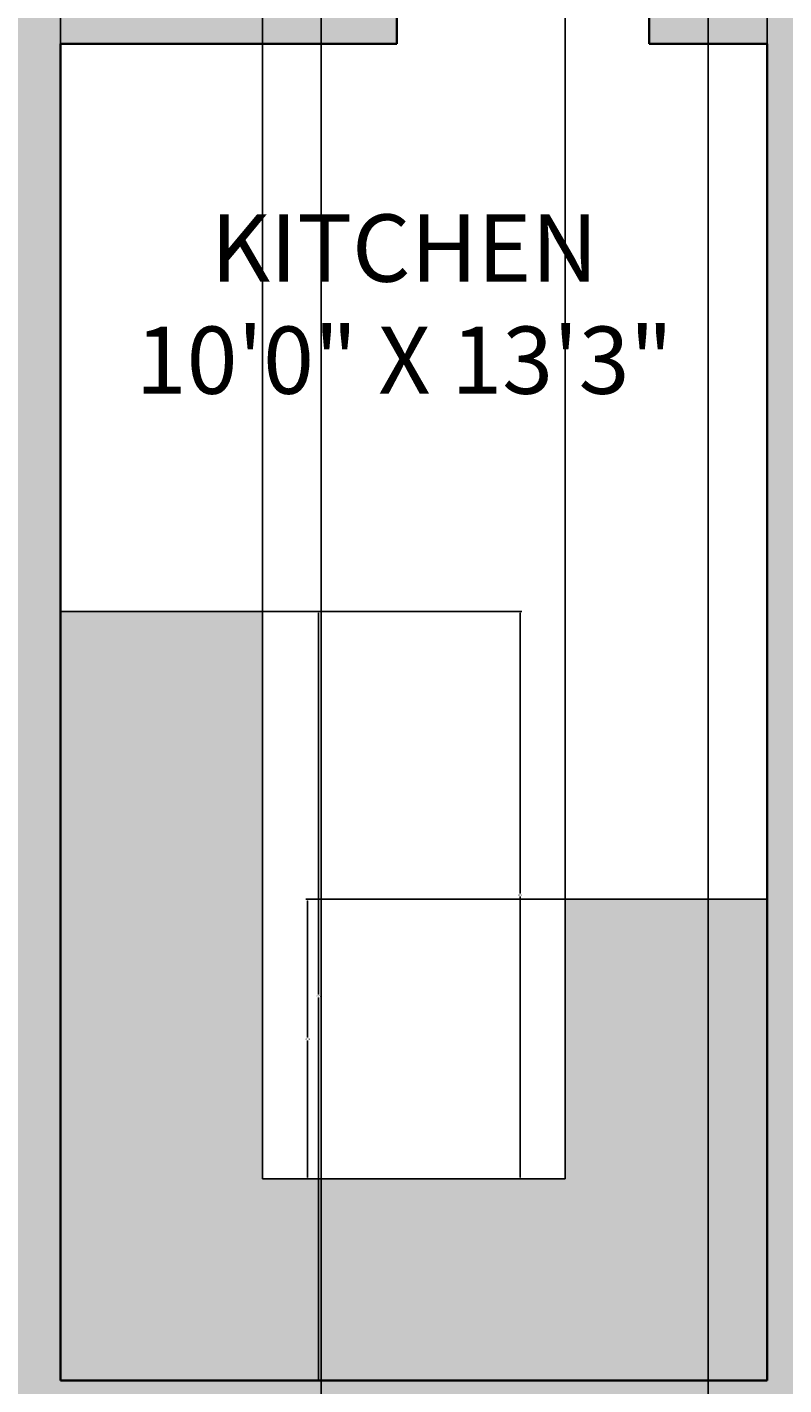
# Model space of a CAD drawing. Units: inches. Extents: x 1567 to 1964, y 1813 to 2447.
# Tile 3 of 28: x 1707 to 1797, y 1964 to 2125. Entities that reach past the tile are written whole.
import ezdxf

# ---------------------------------------------------------------- set-up
doc = ezdxf.new("R2010")
doc.units = ezdxf.units.IN
for name, color, linetype, lineweight in [('A-ANNO-DIMS', 2, 'Continuous', 18), ('A-AREA-IDEN', 7, 'Continuous', 18), ('A-FLOR-CASE', 8, 'Continuous', 25), ('A-WALL', 7, 'Continuous', 35)]:
    doc.layers.add(name, color=color, linetype=linetype, lineweight=lineweight)
doc.layers.add('A-FURN-PATT', color=252, linetype='Continuous', lineweight=13, true_color=0x939598)
doc.layers.add('A-WALL-PATT', color=251, linetype='Continuous', lineweight=13, true_color=0x636466)
doc.styles.get("Standard").update_dxf_attribs({"font": 'arial.ttf'})
doc.dimstyles.get("Standard").update_dxf_attribs({"dimtxt": 0.18, "dimasz": 0.18, "dimexe": 0.18, "dimexo": 0.0625, "dimgap": 0.09, "dimtad": 0, "dimtih": 1, "dimtoh": 1, "dimdec": 4, "dimzin": 0, "dimdsep": 46, "dimtxsty": 'Standard', "dimcen": 0.09, "dimadec": 0, "dimazin": 0, "dimtfac": 1, "dimtdec": 4, "dimtofl": 0, "dimtmove": 0, "dimatfit": 3, "dimfxl": 1, "dimtolj": 1, "dimtzin": 0, "dimarcsym": 0})

# ---------------------------------------------------------------- blocks, each defined once
blk = doc.blocks.new('*D47')
at = {"layer": 'A-ANNO-DIMS', "color": 0, "lineweight": -2, "transparency": 16777216}
for p, q in [((1742.43, 2331.23), (1742.43, 1813.46)), ((1788.43, 2331.23), (1788.43, 1813.46)), ((1742.61, 1813.64), (1765.21, 1813.64)), ((1788.25, 1813.64), (1765.65, 1813.64))]:
    blk.add_line(p, q, dxfattribs=at)
at = {"layer": 'A-ANNO-DIMS', "color": 0, "transparency": 16777216}
for points in [[(1742.61, 1813.67), (1742.61, 1813.61), (1742.43, 1813.64)], [(1788.25, 1813.67), (1788.25, 1813.61), (1788.43, 1813.64)]]:
    blk.add_solid(points, dxfattribs=at)
at = {"layer": 'Defpoints', "color": 0, "transparency": 16777216}
for p in [(1742.43, 2331.29), (1788.43, 2331.29), (1788.43, 1813.64)]:
    blk.add_point(p, dxfattribs=at)
at = {"layer": 'A-ANNO-DIMS', "color": 0, "transparency": 16777216, "insert": (1765.43, 1813.64), "char_height": 0.18, "attachment_point": 5}
blk.add_mtext('\\A1;46', dxfattribs=at)
blk = doc.blocks.new('*D54')
at = {"layer": 'A-ANNO-DIMS', "color": 0, "lineweight": -2, "transparency": 16777216}
for p, q in [((1711.43, 1964.35), (1711.43, 2447.12)), ((1711.61, 2446.94), (1753.21, 2446.94)), ((1795.25, 2446.94), (1753.65, 2446.94)), ((1795.43, 1964.35), (1795.43, 2447.12))]:
    blk.add_line(p, q, dxfattribs=at)
at = {"layer": 'A-ANNO-DIMS', "color": 0, "transparency": 16777216}
for points in [[(1711.61, 2446.97), (1711.61, 2446.91), (1711.43, 2446.94)], [(1795.25, 2446.97), (1795.25, 2446.91), (1795.43, 2446.94)]]:
    blk.add_solid(points, dxfattribs=at)
at = {"layer": 'Defpoints', "color": 0, "transparency": 16777216}
for p in [(1795.43, 2446.94), (1711.43, 1964.29), (1795.43, 1964.29)]:
    blk.add_point(p, dxfattribs=at)
at = {"layer": 'A-ANNO-DIMS', "color": 0, "transparency": 16777216, "insert": (1753.43, 2446.94), "char_height": 0.18, "attachment_point": 5}
blk.add_mtext('\\A1;84', dxfattribs=at)
blk = doc.blocks.new('*D55')
at = {"layer": 'A-ANNO-DIMS', "color": 0, "lineweight": -2, "transparency": 16777216}
for p, q in [((1795.43, 1964.35), (1795.43, 2447.12)), ((1795.61, 2446.94), (1797.28, 2446.94)), ((1799.25, 2446.94), (1797.58, 2446.94)), ((1799.43, 1967.35), (1799.43, 2447.12))]:
    blk.add_line(p, q, dxfattribs=at)
at = {"layer": 'A-ANNO-DIMS', "color": 0, "transparency": 16777216}
for points in [[(1795.61, 2446.97), (1795.61, 2446.91), (1795.43, 2446.94)], [(1799.25, 2446.97), (1799.25, 2446.91), (1799.43, 2446.94)]]:
    blk.add_solid(points, dxfattribs=at)
at = {"layer": 'Defpoints', "color": 0, "transparency": 16777216}
for p in [(1799.43, 2446.94), (1799.43, 1967.29), (1795.43, 1964.29)]:
    blk.add_point(p, dxfattribs=at)
at = {"layer": 'A-ANNO-DIMS', "color": 0, "transparency": 16777216, "insert": (1797.43, 2446.94), "char_height": 0.18, "attachment_point": 5}
blk.add_mtext('\\A1;4', dxfattribs=at)
blk = doc.blocks.new('*D63')
at = {"layer": 'A-ANNO-DIMS', "color": 0, "lineweight": -2, "transparency": 16777216}
for p, q in [((1735.43, 1988.35), (1735.43, 2447.12)), ((1735.61, 2446.94), (1753.21, 2446.94)), ((1771.25, 2446.94), (1753.65, 2446.94)), ((1771.43, 1988.35), (1771.43, 2447.12))]:
    blk.add_line(p, q, dxfattribs=at)
at = {"layer": 'A-ANNO-DIMS', "color": 0, "transparency": 16777216}
for points in [[(1735.61, 2446.97), (1735.61, 2446.91), (1735.43, 2446.94)], [(1771.25, 2446.97), (1771.25, 2446.91), (1771.43, 2446.94)]]:
    blk.add_solid(points, dxfattribs=at)
at = {"layer": 'Defpoints', "color": 0, "transparency": 16777216}
for p in [(1771.43, 2446.94), (1735.43, 1988.29), (1771.43, 1988.29)]:
    blk.add_point(p, dxfattribs=at)
at = {"layer": 'A-ANNO-DIMS', "color": 0, "transparency": 16777216, "insert": (1753.43, 2446.94), "char_height": 0.18, "attachment_point": 5}
blk.add_mtext('\\A1;36', dxfattribs=at)
blk = doc.blocks.new('*D64')
at = {"layer": 'A-ANNO-DIMS', "color": 0, "lineweight": -2, "transparency": 16777216}
for p, q in [((1711.43, 2055.85), (1711.43, 2447.12)), ((1711.61, 2446.94), (1723.21, 2446.94)), ((1735.25, 2446.94), (1723.65, 2446.94)), ((1735.43, 2055.85), (1735.43, 2447.12))]:
    blk.add_line(p, q, dxfattribs=at)
at = {"layer": 'A-ANNO-DIMS', "color": 0, "transparency": 16777216}
for points in [[(1711.61, 2446.97), (1711.61, 2446.91), (1711.43, 2446.94)], [(1735.25, 2446.97), (1735.25, 2446.91), (1735.43, 2446.94)]]:
    blk.add_solid(points, dxfattribs=at)
at = {"layer": 'Defpoints', "color": 0, "transparency": 16777216}
for p in [(1735.43, 2446.94), (1711.43, 2055.79), (1735.43, 2055.79)]:
    blk.add_point(p, dxfattribs=at)
at = {"layer": 'A-ANNO-DIMS', "color": 0, "transparency": 16777216, "insert": (1723.43, 2446.94), "char_height": 0.18, "attachment_point": 5}
blk.add_mtext('\\A1;24', dxfattribs=at)
blk = doc.blocks.new('*D65')
at = {"layer": 'A-ANNO-DIMS', "color": 0, "lineweight": -2, "transparency": 16777216}
for p, q in [((1735.49, 2055.79), (1766.26, 2055.79)), ((1766.08, 2055.61), (1766.08, 2022.22)), ((1766.08, 1988.47), (1766.08, 2021.86)), ((1735.49, 1988.29), (1766.26, 1988.29))]:
    blk.add_line(p, q, dxfattribs=at)
at = {"layer": 'A-ANNO-DIMS', "color": 0, "transparency": 16777216}
for points in [[(1766.05, 2055.61), (1766.11, 2055.61), (1766.08, 2055.79)], [(1766.05, 1988.47), (1766.11, 1988.47), (1766.08, 1988.29)]]:
    blk.add_solid(points, dxfattribs=at)
at = {"layer": 'Defpoints', "color": 0, "transparency": 16777216}
for p in [(1735.43, 2055.79), (1735.43, 1988.29), (1766.08, 1988.29)]:
    blk.add_point(p, dxfattribs=at)
at = {"layer": 'A-ANNO-DIMS', "color": 0, "transparency": 16777216, "insert": (1766.08, 2022.04), "char_height": 0.18, "attachment_point": 5}
blk.add_mtext('\\A1;67.5', dxfattribs=at)
blk = doc.blocks.new('*D66')
at = {"layer": 'A-ANNO-DIMS', "color": 0, "lineweight": -2, "transparency": 16777216}
for p, q in [((1771.37, 2021.55), (1740.6, 2021.55)), ((1740.78, 2021.37), (1740.78, 2005.1)), ((1740.78, 1988.47), (1740.78, 2004.74)), ((1771.37, 1988.29), (1740.6, 1988.29))]:
    blk.add_line(p, q, dxfattribs=at)
at = {"layer": 'A-ANNO-DIMS', "color": 0, "transparency": 16777216}
for points in [[(1740.75, 2021.37), (1740.81, 2021.37), (1740.78, 2021.55)], [(1740.75, 1988.47), (1740.81, 1988.47), (1740.78, 1988.29)]]:
    blk.add_solid(points, dxfattribs=at)
at = {"layer": 'Defpoints', "color": 0, "transparency": 16777216}
for p in [(1740.78, 2021.55), (1771.43, 2021.55), (1771.43, 1988.29)]:
    blk.add_point(p, dxfattribs=at)
at = {"layer": 'A-ANNO-DIMS', "color": 0, "transparency": 16777216, "insert": (1740.78, 2004.92), "char_height": 0.18, "attachment_point": 5}
blk.add_mtext('\\A1;33.26', dxfattribs=at)
blk = doc.blocks.new('*D67')
at = {"layer": 'A-ANNO-DIMS', "color": 0, "lineweight": -2, "transparency": 16777216}
for p, q in [((1711.49, 2055.79), (1742.26, 2055.79)), ((1742.08, 2055.61), (1742.08, 2010.22)), ((1742.08, 1964.47), (1742.08, 2009.86)), ((1711.49, 1964.29), (1742.26, 1964.29))]:
    blk.add_line(p, q, dxfattribs=at)
at = {"layer": 'A-ANNO-DIMS', "color": 0, "transparency": 16777216}
for points in [[(1742.05, 2055.61), (1742.11, 2055.61), (1742.08, 2055.79)], [(1742.05, 1964.47), (1742.11, 1964.47), (1742.08, 1964.29)]]:
    blk.add_solid(points, dxfattribs=at)
at = {"layer": 'Defpoints', "color": 0, "transparency": 16777216}
for p in [(1711.43, 2055.79), (1711.43, 1964.29), (1742.08, 1964.29)]:
    blk.add_point(p, dxfattribs=at)
at = {"layer": 'A-ANNO-DIMS', "color": 0, "transparency": 16777216, "insert": (1742.08, 2010.04), "char_height": 0.18, "attachment_point": 5}
blk.add_mtext('\\A1;91.5', dxfattribs=at)

msp = doc.modelspace()

# ---------------------------------------------------------------- hatches: boundary and pattern name
at = {"layer": 'A-FURN-PATT'}
h = msp.add_hatch(color=256, dxfattribs=at)
h.dxf.hatch_style = 1
h.paths.add_polyline_path([(1697.3402, 2374.8316), (1682.1402, 2374.8316), (1682.1402, 2387.6316), (1637.3402, 2387.6316), (1637.3402, 2324.4315), (1697.3402, 2324.4315)])
h.paths.add_polyline_path([(1891.1093, 2375.8204), (1875.9094, 2375.8204), (1875.9094, 2388.6204), (1831.1094, 2388.6204), (1831.1094, 2325.4204), (1891.1093, 2325.4204)])
h.paths.add_polyline_path([(1702.5611, 2206.8057), (1702.5611, 2210.8057), (1699.7395, 2209.9436), (1697.013, 2209.2403), (1694.3857, 2208.6763), (1691.8615, 2208.2326), (1689.4443, 2207.8896), (1687.1381, 2207.6282), (1684.9469, 2207.4289), (1682.8747, 2207.2725), (1680.9233, 2207.1425), (1679.0865, 2207.0339), (1677.3558, 2206.9445), (1675.7229, 2206.8719), (1674.1794, 2206.8141), (1672.7169, 2206.7688), (1671.327, 2206.7339), (1670.0014, 2206.707), (1668.7314, 2206.6866), (1667.5072, 2206.6732), (1666.3188, 2206.668), (1665.1561, 2206.6722), (1664.009, 2206.6869), (1662.8675, 2206.7133), (1661.7215, 2206.7525), (1660.5611, 2206.8057), (1660.5611, 2202.8057), (1661.9932, 2202.9556), (1663.3314, 2203.0744), (1664.5899, 2203.1671), (1665.7831, 2203.2385), (1666.9254, 2203.2935), (1668.0311, 2203.3368), (1669.1145, 2203.3734), (1670.1902, 2203.4081), (1671.2724, 2203.4451), (1672.3759, 2203.4866), (1673.5155, 2203.534), (1674.706, 2203.5887), (1675.9621, 2203.6523), (1677.2986, 2203.7262), (1678.7304, 2203.8118), (1680.2722, 2203.9108), (1681.947, 2204.0272), (1683.8108, 2204.1769), (1685.9279, 2204.3782), (1688.3626, 2204.6496), (1691.179, 2205.0096), (1694.4413, 2205.4767), (1698.214, 2206.0692)])
h.paths.add_polyline_path([(1702.5611, 2218.8057), (1701.9821, 2217.9383), (1701.3316, 2217.191), (1700.6091, 2216.5515), (1699.8141, 2216.0071), (1698.946, 2215.5454), (1698.0041, 2215.1536), (1696.9879, 2214.8194), (1695.8969, 2214.5301), (1694.7328, 2214.2753), (1693.5072, 2214.0522), (1692.2339, 2213.8602), (1690.9266, 2213.6989), (1689.5994, 2213.5675), (1688.266, 2213.4654), (1686.9402, 2213.392), (1685.636, 2213.3467), (1684.3619, 2213.3287), (1683.1053, 2213.3361), (1681.8482, 2213.3668), (1680.5727, 2213.4187), (1679.2608, 2213.4898), (1677.8948, 2213.5779), (1676.4565, 2213.6811), (1674.9282, 2213.7971), (1673.2982, 2213.9236), (1671.5804, 2214.0573), (1669.795, 2214.1945), (1667.9622, 2214.3316), (1666.1022, 2214.4649), (1664.2352, 2214.5908), (1662.3814, 2214.7056), (1660.5611, 2214.8057), (1660.5611, 2206.8057), (1661.7215, 2206.7525), (1662.8675, 2206.7133), (1664.009, 2206.6869), (1665.1561, 2206.6722), (1666.3188, 2206.668), (1667.5072, 2206.6732), (1668.7314, 2206.6866), (1670.0014, 2206.707), (1671.327, 2206.7339), (1672.7169, 2206.7688), (1674.1794, 2206.8141), (1675.7229, 2206.8719), (1677.3558, 2206.9445), (1679.0865, 2207.0339), (1680.9233, 2207.1425), (1682.8747, 2207.2725), (1684.9469, 2207.4289), (1687.1381, 2207.6282), (1689.4443, 2207.8896), (1691.8615, 2208.2326), (1694.3857, 2208.6763), (1697.013, 2209.2403), (1699.7395, 2209.9436), (1702.5611, 2210.8057)])
h.paths.add_polyline_path([(1700.6091, 2216.5515), (1701.3316, 2217.191), (1701.9821, 2217.9383), (1702.5611, 2218.8057), (1702.5611, 2222.8057), (1689.452, 2222.8057), (1689.0171, 2222.4556), (1688.4521, 2222.0354), (1687.7806, 2221.5662), (1687.0235, 2221.067), (1686.2019, 2220.5566), (1685.3367, 2220.0541), (1684.4491, 2219.5785), (1683.56, 2219.1486), (1682.6867, 2218.7795), (1681.8312, 2218.4692), (1680.9918, 2218.212), (1680.1667, 2218.0019), (1679.3541, 2217.833), (1678.5524, 2217.6995), (1677.7597, 2217.5954), (1676.9744, 2217.5149), (1676.1942, 2217.4531), (1675.4146, 2217.4093), (1674.6309, 2217.384), (1673.8381, 2217.3774), (1673.0313, 2217.39), (1672.2056, 2217.4221), (1671.3562, 2217.4741), (1670.4782, 2217.5463), (1669.5642, 2217.639), (1668.5968, 2217.7516), (1667.5562, 2217.8833), (1666.4226, 2218.0336), (1665.1761, 2218.2017), (1663.7969, 2218.3869), (1662.2651, 2218.5885), (1660.5611, 2218.8057), (1660.5611, 2214.8057), (1662.3814, 2214.7056), (1664.2352, 2214.5908), (1666.1022, 2214.4649), (1667.9622, 2214.3316), (1669.795, 2214.1945), (1671.5804, 2214.0573), (1673.2982, 2213.9236), (1674.9282, 2213.7971), (1676.4565, 2213.6811), (1677.8948, 2213.5779), (1679.2608, 2213.4898), (1680.5727, 2213.4187), (1681.8482, 2213.3668), (1683.1053, 2213.3361), (1684.3619, 2213.3287), (1685.636, 2213.3467), (1686.9402, 2213.392), (1688.266, 2213.4654), (1689.5994, 2213.5675), (1690.9266, 2213.6989), (1692.2339, 2213.8602), (1693.5072, 2214.0522), (1694.7328, 2214.2753), (1695.8969, 2214.5301), (1696.9879, 2214.8194), (1698.0041, 2215.1536), (1698.946, 2215.5454), (1699.8141, 2216.0071)])
h.paths.add_polyline_path([(1687.0235, 2221.067), (1687.7806, 2221.5662), (1688.4521, 2222.0354), (1689.0171, 2222.4556), (1689.452, 2222.8057), (1660.5611, 2222.8057), (1660.5611, 2218.8057), (1662.2651, 2218.5885), (1663.7969, 2218.3869), (1665.1761, 2218.2017), (1666.4226, 2218.0336), (1667.5562, 2217.8833), (1668.5968, 2217.7516), (1669.5642, 2217.639), (1670.4782, 2217.5463), (1671.3562, 2217.4741), (1672.2056, 2217.4221), (1673.0313, 2217.39), (1673.8381, 2217.3774), (1674.6309, 2217.384), (1675.4146, 2217.4093), (1676.1942, 2217.4531), (1676.9744, 2217.5149), (1677.7597, 2217.5954), (1678.5524, 2217.6995), (1679.3541, 2217.833), (1680.1667, 2218.0019), (1680.9918, 2218.212), (1681.8312, 2218.4692), (1682.6867, 2218.7795), (1683.56, 2219.1486), (1684.4491, 2219.5785), (1685.3367, 2220.0541), (1686.2019, 2220.5566)], flags=17)
h.paths.add_polyline_path([(1702.5611, 2198.8057), (1698.9289, 2199.2412), (1695.8472, 2199.5774), (1693.2166, 2199.8257), (1690.9377, 2199.9973), (1688.9111, 2200.1033), (1687.0375, 2200.155), (1685.2174, 2200.1637), (1683.3514, 2200.1406), (1681.3514, 2200.0941), (1679.1736, 2200.0225), (1676.7858, 2199.921), (1674.1554, 2199.7852), (1671.2502, 2199.6103), (1668.0377, 2199.3919), (1664.4854, 2199.1252), (1660.5611, 2198.8057), (1660.5611, 2194.8057), (1662.2697, 2194.9771), (1663.9673, 2195.0999), (1665.6339, 2195.1809), (1667.2495, 2195.227), (1668.7941, 2195.2449), (1670.2478, 2195.2414), (1671.5906, 2195.2233), (1672.8026, 2195.1974), (1673.8739, 2195.1689), (1674.8359, 2195.1364), (1675.7302, 2195.0967), (1676.5982, 2195.0469), (1677.4817, 2194.9838), (1678.422, 2194.9043), (1679.4609, 2194.8055), (1680.6397, 2194.6842), (1682.005, 2194.5341), (1683.6223, 2194.335), (1685.562, 2194.0637), (1687.8945, 2193.6967), (1690.6902, 2193.2108), (1694.0196, 2192.5826), (1697.9531, 2191.7887), (1702.5611, 2190.8057)])
h.paths.add_polyline_path([(1702.5611, 2206.8057), (1698.214, 2206.0692), (1694.4413, 2205.4767), (1691.179, 2205.0096), (1688.3626, 2204.6496), (1685.9279, 2204.3782), (1683.8108, 2204.1769), (1681.947, 2204.0272), (1680.2722, 2203.9108), (1678.7304, 2203.8118), (1677.2986, 2203.7262), (1675.9621, 2203.6523), (1674.706, 2203.5887), (1673.5155, 2203.534), (1672.3759, 2203.4866), (1671.2724, 2203.4451), (1670.1902, 2203.4081), (1669.1145, 2203.3734), (1668.0311, 2203.3368), (1666.9254, 2203.2935), (1665.7831, 2203.2385), (1664.5899, 2203.1671), (1663.3314, 2203.0744), (1661.9932, 2202.9556), (1660.5611, 2202.8057), (1660.5611, 2198.8057), (1664.4854, 2199.1252), (1668.0377, 2199.3919), (1671.2502, 2199.6103), (1674.1554, 2199.7852), (1676.7858, 2199.921), (1679.1736, 2200.0225), (1681.3514, 2200.0941), (1683.3514, 2200.1406), (1685.2174, 2200.1637), (1687.0375, 2200.155), (1688.9111, 2200.1033), (1690.9377, 2199.9973), (1693.2166, 2199.8257), (1695.8472, 2199.5774), (1698.9289, 2199.2412), (1702.5611, 2198.8057)])
h.paths.add_polyline_path([(1702.5611, 2190.8057), (1697.9531, 2191.7887), (1694.0196, 2192.5826), (1690.6902, 2193.2108), (1687.8945, 2193.6967), (1685.562, 2194.0637), (1683.6223, 2194.335), (1682.005, 2194.5341), (1680.6397, 2194.6842), (1679.4609, 2194.8055), (1678.422, 2194.9043), (1677.4817, 2194.9838), (1676.5982, 2195.0469), (1675.7302, 2195.0967), (1674.8359, 2195.1364), (1673.8739, 2195.1689), (1672.8026, 2195.1974), (1671.5906, 2195.2233), (1670.2478, 2195.2414), (1668.7941, 2195.2449), (1667.2495, 2195.227), (1665.6339, 2195.1809), (1663.9673, 2195.0999), (1662.2697, 2194.9771), (1660.5611, 2194.8057), (1660.5611, 2190.8057), (1665.9637, 2190.2699), (1670.5105, 2189.7867), (1674.3035, 2189.3504), (1677.4445, 2188.9552), (1680.0354, 2188.5951), (1682.1782, 2188.2644), (1683.9747, 2187.9571), (1685.5268, 2187.6675), (1686.9225, 2187.3901), (1688.1943, 2187.1216), (1689.3606, 2186.859), (1690.4399, 2186.5993), (1691.4508, 2186.3396), (1692.4118, 2186.0769), (1693.3413, 2185.8084), (1694.2579, 2185.531), (1695.1786, 2185.2422), (1696.1142, 2184.9406), (1697.0739, 2184.6252), (1698.0671, 2184.2949), (1699.1032, 2183.9489), (1700.1913, 2183.586), (1701.3408, 2183.2053), (1702.5611, 2182.8057)])
h.paths.add_polyline_path([(1702.5611, 2182.8057), (1701.3408, 2183.2053), (1700.1913, 2183.586), (1699.1032, 2183.9489), (1698.0671, 2184.2949), (1697.0739, 2184.6252), (1696.1142, 2184.9406), (1695.1786, 2185.2422), (1694.2579, 2185.531), (1693.3413, 2185.8084), (1692.4118, 2186.0769), (1691.4508, 2186.3396), (1690.4399, 2186.5993), (1689.3606, 2186.859), (1688.1943, 2187.1216), (1686.9225, 2187.3901), (1685.5268, 2187.6675), (1683.9747, 2187.9571), (1682.1782, 2188.2644), (1680.0354, 2188.5951), (1677.4445, 2188.9552), (1674.3035, 2189.3504), (1670.5105, 2189.7867), (1665.9637, 2190.2699), (1660.5611, 2190.8057), (1660.5611, 2186.8057), (1663.5709, 2186.52), (1666.0965, 2186.2414), (1668.1979, 2185.9698), (1669.9351, 2185.7048), (1671.3681, 2185.446), (1672.5568, 2185.1931), (1673.5613, 2184.9458), (1674.4415, 2184.7037), (1675.2485, 2184.4664), (1675.9976, 2184.2328), (1677.0295, 2183.8907), (1678.2492, 2183.4332), (1679.354, 2182.9669), (1680.4123, 2182.4724), (1681.3757, 2181.9718), (1682.2435, 2181.4594), (1683.1864, 2180.8057), (1702.5611, 2180.8057)])
h.paths.add_polyline_path([(1677.3469, 2183.7716), (1676.6949, 2184.0016), (1675.9976, 2184.2328), (1675.2485, 2184.4664), (1674.4415, 2184.7037), (1673.5613, 2184.9458), (1672.5568, 2185.1931), (1671.3681, 2185.446), (1669.9351, 2185.7048), (1668.1979, 2185.9698), (1666.0965, 2186.2414), (1663.5709, 2186.52), (1660.5611, 2186.8057), (1660.5611, 2180.8057), (1683.1506, 2180.8057), (1682.802, 2181.0722), (1682.4264, 2181.3326), (1682.0201, 2181.5913), (1681.586, 2181.8476), (1681.1268, 2182.1011), (1680.6453, 2182.3513), (1680.1443, 2182.5976), (1679.6266, 2182.8395), (1679.0933, 2183.0769), (1678.5398, 2183.3105), (1677.9598, 2183.5417)], flags=17)
h.paths.add_polyline_path([(1824.4511, 2199.9016), (1824.089, 2199.9302), (1824.0595, 2199.9372), (1824.0397, 2199.9406), (1823.5413, 2200.0576), (1823.4095, 2200.0864), (1823.0664, 2200.1559), (1822.6419, 2200.2361), (1822.1519, 2200.3222), (1821.6126, 2200.4093), (1821.0401, 2200.4925), (1820.4505, 2200.5669), (1819.8599, 2200.6276), (1819.2845, 2200.6697), (1818.7366, 2200.6896), (1818.2141, 2200.688), (1817.7112, 2200.6668), (1817.222, 2200.6281), (1816.7405, 2200.5737), (1816.261, 2200.5057), (1815.7776, 2200.4259), (1815.2845, 2200.3364), (1814.3007, 2200.149), (1813.3315, 2199.9765), (1812.406, 2199.8514), (1811.6868, 2199.7739), (1810.8992, 2199.7121), (1810.0345, 2199.6697), (1809.0854, 2199.6497), (1808.0514, 2199.6502), (1806.9334, 2199.6683), (1805.7324, 2199.701), (1804.4493, 2199.7454), (1803.0852, 2199.7986), (1801.641, 2199.8577), (1800.1178, 2199.9197), (1798.5134, 2199.9818), (1796.8144, 2200.0415), (1795.004, 2200.0962), (1793.0657, 2200.1437), (1790.9828, 2200.1814), (1788.7389, 2200.2068), (1786.3171, 2200.2177), (1783.7011, 2200.2114), (1780.8715, 2200.185), (1777.7988, 2200.1326), (1774.4506, 2200.0481), (1770.7948, 2199.9249), (1766.7992, 2199.7569), (1762.4316, 2199.5376), (1757.6596, 2199.2606), (1752.4511, 2198.9197), (1752.4511, 2193.4197), (1761.2668, 2193.6071), (1768.3671, 2193.7934), (1773.9821, 2193.9778), (1778.3417, 2194.1593), (1781.6759, 2194.3369), (1784.2148, 2194.5096), (1786.1882, 2194.6764), (1787.8261, 2194.8364), (1789.3219, 2194.9887), (1790.7226, 2195.1333), (1792.0383, 2195.27), (1793.2792, 2195.3989), (1794.4557, 2195.52), (1795.5781, 2195.6333), (1796.6564, 2195.7387), (1797.7011, 2195.8364), (1798.7216, 2195.9259), (1799.7245, 2196.0057), (1800.7158, 2196.0737), (1801.7011, 2196.1281), (1802.6865, 2196.1668), (1803.6777, 2196.188), (1804.6806, 2196.1896), (1805.7011, 2196.1697), (1806.7423, 2196.1273), (1807.7962, 2196.0643), (1808.852, 2195.9837), (1809.899, 2195.8885), (1810.9265, 2195.7815), (1811.9238, 2195.6658), (1812.88, 2195.5442), (1813.7845, 2195.4197), (1814.6296, 2195.2948), (1815.4205, 2195.1704), (1816.1656, 2195.0469), (1816.873, 2194.9249), (1817.5511, 2194.8049), (1818.2083, 2194.6873), (1818.8527, 2194.5726), (1819.4928, 2194.4614), (1820.1348, 2194.3554), (1820.7773, 2194.2615), (1821.4169, 2194.1882), (1822.0501, 2194.1437), (1822.6735, 2194.1363), (1823.2838, 2194.1743), (1823.8775, 2194.266), (1824.4511, 2194.4197)])
h.paths.add_polyline_path([(1821.4716, 2190.5098), (1820.4303, 2190.5708), (1819.3811, 2190.6415), (1818.3339, 2190.7186), (1817.2985, 2190.7986), (1816.2845, 2190.8781), (1815.2976, 2190.9542), (1814.3274, 2191.0259), (1813.3592, 2191.0927), (1812.3782, 2191.1541), (1811.3699, 2191.2097), (1810.3196, 2191.2589), (1809.2127, 2191.3013), (1808.0345, 2191.3364), (1806.7708, 2191.3634), (1805.4094, 2191.3807), (1803.9387, 2191.3862), (1802.3469, 2191.3781), (1800.6223, 2191.3543), (1798.7532, 2191.313), (1796.7278, 2191.2521), (1794.5344, 2191.1697), (1792.128, 2191.0648), (1789.33, 2190.9393), (1785.9285, 2190.7962), (1781.7115, 2190.6385), (1776.4672, 2190.469), (1769.9836, 2190.2908), (1762.0489, 2190.1067), (1752.4511, 2189.9197), (1752.4511, 2185.4197), (1758.363, 2185.5846), (1763.4179, 2185.7075), (1767.7199, 2185.7933), (1771.373, 2185.8468), (1774.4811, 2185.873), (1777.1484, 2185.8768), (1779.4787, 2185.8629), (1781.5761, 2185.8364), (1783.5287, 2185.8014), (1785.3606, 2185.7596), (1787.0802, 2185.7119), (1788.6959, 2185.6593), (1790.2158, 2185.6028), (1791.6484, 2185.5434), (1793.0018, 2185.4821), (1794.2844, 2185.4197), (1795.5065, 2185.3576), (1796.6861, 2185.298), (1797.8433, 2185.2432), (1798.998, 2185.1958), (1800.1703, 2185.1581), (1801.3801, 2185.1326), (1802.6476, 2185.1218), (1803.9928, 2185.1281), (1805.4444, 2185.1555), (1807.0663, 2185.2147), (1808.9315, 2185.3178), (1811.1126, 2185.477), (1813.6823, 2185.7046), (1816.7135, 2186.0128), (1820.2788, 2186.4138), (1824.4511, 2186.9197), (1824.4511, 2190.4197), (1823.4918, 2190.4309), (1822.4954, 2190.4621)])
h.paths.add_polyline_path([(1797.3762, 2216.0584), (1797.6199, 2216.2267), (1797.9558, 2216.3355), (1798.3017, 2216.3703), (1798.5761, 2216.3781), (1798.8974, 2216.3703), (1799.2714, 2216.3468), (1799.704, 2216.3078), (1800.2011, 2216.2531), (1800.7695, 2216.1829), (1801.4205, 2216.0981), (1802.1662, 2215.9996), (1803.0188, 2215.8885), (1803.9906, 2215.7656), (1805.0937, 2215.632), (1806.3404, 2215.4886), (1807.7428, 2215.3364), (1809.3101, 2215.1764), (1811.039, 2215.0096), (1812.9232, 2214.8369), (1814.9563, 2214.6593), (1817.132, 2214.4778), (1819.444, 2214.2934), (1821.8858, 2214.1071), (1824.4511, 2213.9197), (1824.4511, 2217.9197), (1752.4511, 2217.9197), (1752.4511, 2214.9197), (1757.2739, 2214.8973), (1761.6432, 2214.8338), (1765.5973, 2214.7352), (1769.1751, 2214.6072), (1772.4149, 2214.4559), (1775.3554, 2214.2869), (1778.0352, 2214.1063), (1780.4928, 2213.9197), (1782.7607, 2213.7329), (1784.8476, 2213.5499), (1786.7557, 2213.3748), (1788.4876, 2213.2114), (1790.0456, 2213.0636), (1791.4322, 2212.9354), (1792.6499, 2212.8305), (1793.7011, 2212.7531), (1794.5904, 2212.7059), (1795.3313, 2212.688), (1795.9394, 2212.6974), (1796.4303, 2212.7322), (1796.8196, 2212.7905), (1797.123, 2212.8703), (1797.356, 2212.9695), (1797.5344, 2213.0864), (1797.6716, 2213.2187), (1797.7727, 2213.3637), (1797.8406, 2213.5185), (1797.8782, 2213.6801), (1797.8884, 2213.8457), (1797.8743, 2214.0122), (1797.8386, 2214.1767), (1797.7844, 2214.3364), (1797.7149, 2214.4889), (1797.6347, 2214.6346), (1797.5486, 2214.7744), (1797.3327, 2215.109), (1797.178, 2215.4303), (1797.1896, 2215.7939)])
h.paths.add_polyline_path([(1804.7872, 2210.6789), (1804.546, 2211.022), (1804.3512, 2211.3917), (1804.2466, 2211.7546), (1804.2574, 2212.0998), (1804.4058, 2212.4178), (1804.7068, 2212.7007), (1805.1359, 2212.9124), (1805.5279, 2212.9926), (1805.8136, 2213.0154), (1806.1178, 2213.0031), (1806.4405, 2212.9529), (1806.7929, 2212.867), (1807.1893, 2212.7489), (1807.6438, 2212.602), (1808.1706, 2212.4297), (1808.7838, 2212.2355), (1809.4976, 2212.0227), (1810.3261, 2211.7947), (1811.2868, 2211.5533), (1812.4101, 2211.2928), (1813.7297, 2211.0059), (1815.2793, 2210.6854), (1817.0925, 2210.3238), (1819.2031, 2209.9139), (1821.6447, 2209.4483), (1824.4511, 2208.9197), (1824.4511, 2213.9197), (1821.8858, 2214.1071), (1819.444, 2214.2934), (1817.132, 2214.4778), (1814.9563, 2214.6593), (1812.9232, 2214.8369), (1811.039, 2215.0096), (1809.3101, 2215.1764), (1807.7428, 2215.3364), (1806.3404, 2215.4886), (1805.0937, 2215.632), (1803.9906, 2215.7656), (1803.0188, 2215.8885), (1802.1662, 2215.9996), (1801.4205, 2216.0981), (1800.7695, 2216.1829), (1800.2011, 2216.2531), (1799.704, 2216.3078), (1799.2714, 2216.3468), (1798.8974, 2216.3703), (1798.5761, 2216.3781), (1798.3017, 2216.3703), (1798.0683, 2216.3468), (1797.87, 2216.3078), (1797.7011, 2216.2531), (1797.5566, 2216.1831), (1797.4355, 2216.0994), (1797.3378, 2216.004), (1797.2636, 2215.8989), (1797.2128, 2215.7859), (1797.1855, 2215.6671), (1797.1816, 2215.5444), (1797.2011, 2215.4197), (1797.2433, 2215.2946), (1797.304, 2215.1684), (1797.3783, 2215.0403), (1797.4615, 2214.9093), (1797.6718, 2214.5836), (1797.8218, 2214.2545), (1797.8933, 2213.9247), (1797.8728, 2213.5918), (1797.7366, 2213.2814), (1797.4586, 2213.0132), (1797.123, 2212.8703), (1796.8196, 2212.7905), (1796.4303, 2212.7322), (1795.9394, 2212.6974), (1795.3313, 2212.688), (1794.5904, 2212.7059), (1793.7011, 2212.7531), (1792.6499, 2212.8305), (1791.4322, 2212.9354), (1790.0456, 2213.0636), (1788.4876, 2213.2114), (1786.7557, 2213.3748), (1784.8476, 2213.5499), (1782.7607, 2213.7329), (1780.4928, 2213.9197), (1778.0352, 2214.1063), (1775.3554, 2214.2869), (1772.4149, 2214.4559), (1769.1751, 2214.6072), (1765.5973, 2214.7352), (1761.6432, 2214.8338), (1757.2739, 2214.8973), (1752.4511, 2214.9197), (1752.4511, 2209.9197), (1759.4745, 2210.0625), (1765.2786, 2210.1242), (1770.027, 2210.1175), (1773.8834, 2210.0551), (1777.0112, 2209.9498), (1779.5741, 2209.8143), (1781.7357, 2209.6611), (1783.6594, 2209.5031), (1785.4813, 2209.3506), (1787.2265, 2209.2049), (1788.8926, 2209.0651), (1790.4771, 2208.9301), (1791.9777, 2208.7991), (1793.3919, 2208.671), (1794.7171, 2208.5449), (1795.9511, 2208.4197), (1797.0922, 2208.2952), (1798.1425, 2208.1736), (1799.1049, 2208.0579), (1799.9823, 2207.951), (1800.7778, 2207.8558), (1801.4941, 2207.7752), (1802.1342, 2207.7122), (1802.7011, 2207.6697), (1803.1982, 2207.65), (1803.6308, 2207.6528), (1804.0048, 2207.6771), (1804.3261, 2207.7218), (1804.6005, 2207.7861), (1804.8339, 2207.869), (1805.0322, 2207.9694), (1805.2011, 2208.0864), (1805.3455, 2208.2189), (1805.4654, 2208.365), (1805.56, 2208.5229), (1805.6282, 2208.6906), (1805.6691, 2208.866), (1805.6816, 2209.0473), (1805.6648, 2209.2326), (1805.6178, 2209.4197), (1805.5406, 2209.6072), (1805.4381, 2209.7947), (1805.316, 2209.9822), (1805.1803, 2210.1697), (1805.0367, 2210.3572)])
h.paths.add_polyline_path([(1801.4941, 2207.7752), (1800.7778, 2207.8558), (1799.9823, 2207.951), (1799.1049, 2208.0579), (1798.1425, 2208.1736), (1797.0922, 2208.2952), (1795.9511, 2208.4197), (1794.7171, 2208.5449), (1793.3919, 2208.671), (1791.9777, 2208.7991), (1790.4771, 2208.9301), (1788.8926, 2209.0651), (1787.2265, 2209.2049), (1785.4813, 2209.3506), (1783.6594, 2209.5031), (1781.7357, 2209.6611), (1779.5741, 2209.8143), (1777.0112, 2209.9498), (1773.8834, 2210.0551), (1770.027, 2210.1175), (1765.2786, 2210.1242), (1759.4745, 2210.0625), (1752.4511, 2209.9197), (1752.4511, 2205.4197), (1757.7354, 2205.2545), (1762.3821, 2205.1294), (1766.4565, 2205.0374), (1770.024, 2204.9718), (1773.1502, 2204.9258), (1775.9003, 2204.8924), (1778.3399, 2204.8649), (1780.5344, 2204.8364), (1782.5421, 2204.8014), (1784.3925, 2204.7596), (1786.1082, 2204.7119), (1787.7115, 2204.6593), (1789.225, 2204.6028), (1790.6711, 2204.5434), (1792.0724, 2204.4821), (1793.4511, 2204.4197), (1794.8241, 2204.3576), (1796.1855, 2204.2973), (1797.5234, 2204.241), (1798.8261, 2204.1906), (1800.082, 2204.1479), (1801.2792, 2204.115), (1802.4062, 2204.0939), (1803.4511, 2204.0864), (1804.4051, 2204.0942), (1805.2701, 2204.1176), (1806.0512, 2204.1567), (1806.7532, 2204.2114), (1807.381, 2204.2817), (1807.9394, 2204.3676), (1808.4334, 2204.4692), (1808.8678, 2204.5864), (1809.248, 2204.7187), (1809.5813, 2204.8637), (1809.8756, 2205.0185), (1810.1386, 2205.1801), (1810.3782, 2205.3457), (1810.6022, 2205.5122), (1810.9725, 2205.7941), (1811.3803, 2206.072), (1811.739, 2206.2612), (1812.0032, 2206.3781), (1812.2869, 2206.4793), (1812.5931, 2206.563), (1812.9246, 2206.6271), (1813.2845, 2206.6697), (1813.6746, 2206.6894), (1814.0931, 2206.6867), (1814.5369, 2206.6624), (1815.0032, 2206.6176), (1815.489, 2206.5534), (1815.9915, 2206.4705), (1816.5076, 2206.3701), (1817.0345, 2206.2531), (1817.5753, 2206.1196), (1818.1582, 2205.9666), (1818.8172, 2205.7902), (1819.5865, 2205.5864), (1820.5004, 2205.3514), (1821.5931, 2205.0812), (1822.8986, 2204.7719), (1824.4511, 2204.4197), (1824.4511, 2208.9197), (1821.6447, 2209.4483), (1819.2031, 2209.9139), (1817.0925, 2210.3238), (1815.2793, 2210.6854), (1813.7297, 2211.0059), (1812.4101, 2211.2928), (1811.2868, 2211.5533), (1810.3261, 2211.7947), (1809.4976, 2212.0227), (1808.7838, 2212.2355), (1808.1706, 2212.4297), (1807.6438, 2212.602), (1807.1893, 2212.7489), (1806.7929, 2212.867), (1806.4405, 2212.9529), (1806.1178, 2213.0031), (1805.8136, 2213.0154), (1805.5279, 2212.9926), (1805.2638, 2212.9386), (1805.024, 2212.8572), (1804.8116, 2212.7524), (1804.6295, 2212.6281), (1804.4806, 2212.4881), (1804.3678, 2212.3364), (1804.2931, 2212.1764), (1804.2545, 2212.0096), (1804.2491, 2211.8369), (1804.274, 2211.6593), (1804.3263, 2211.4778), (1804.4029, 2211.2934), (1804.5011, 2211.1071), (1804.6178, 2210.9197), (1804.7496, 2210.7322), (1804.8912, 2210.5447), (1805.154, 2210.2061), (1805.3962, 2209.8715), (1805.5964, 2209.5053), (1805.688, 2209.1402), (1805.6629, 2208.7758), (1805.5257, 2208.4385), (1805.2839, 2208.1437), (1804.9434, 2207.9078), (1804.6005, 2207.7861), (1804.3261, 2207.7218), (1804.0048, 2207.6771), (1803.6308, 2207.6528), (1803.1982, 2207.65), (1802.7011, 2207.6697), (1802.1342, 2207.7122)])
h.paths.add_polyline_path([(1824.4511, 2204.4197), (1822.8986, 2204.7719), (1821.5931, 2205.0812), (1820.5004, 2205.3514), (1819.5865, 2205.5864), (1818.8172, 2205.7902), (1818.1582, 2205.9666), (1817.5753, 2206.1196), (1817.0345, 2206.2531), (1816.5076, 2206.3701), (1815.9915, 2206.4705), (1815.489, 2206.5534), (1815.0032, 2206.6176), (1814.5369, 2206.6624), (1814.0931, 2206.6867), (1813.6746, 2206.6894), (1813.2845, 2206.6697), (1812.9246, 2206.6271), (1812.5931, 2206.563), (1812.2869, 2206.4793), (1812.0032, 2206.3781), (1811.739, 2206.2612), (1811.4915, 2206.1307), (1811.2576, 2205.9884), (1811.0345, 2205.8364), (1810.8183, 2205.6767), (1810.4357, 2205.3854), (1810.1386, 2205.1801), (1809.8756, 2205.0185), (1809.5813, 2204.8637), (1809.248, 2204.7187), (1808.8678, 2204.5864), (1808.4334, 2204.4692), (1807.9394, 2204.3676), (1807.381, 2204.2817), (1806.7532, 2204.2114), (1806.0512, 2204.1567), (1805.2701, 2204.1176), (1804.4051, 2204.0942), (1803.4511, 2204.0864), (1802.4062, 2204.0939), (1801.2792, 2204.115), (1800.082, 2204.1479), (1798.8261, 2204.1906), (1797.5234, 2204.241), (1796.1855, 2204.2973), (1794.8241, 2204.3576), (1793.4511, 2204.4197), (1792.0724, 2204.4821), (1790.6711, 2204.5434), (1789.225, 2204.6028), (1787.7115, 2204.6593), (1786.1082, 2204.7119), (1784.3925, 2204.7596), (1782.5421, 2204.8014), (1780.5344, 2204.8364), (1778.3399, 2204.8649), (1775.9003, 2204.8924), (1773.1502, 2204.9258), (1770.024, 2204.9718), (1766.4565, 2205.0374), (1762.3821, 2205.1294), (1757.7354, 2205.2545), (1752.4511, 2205.4197), (1752.4511, 2198.9197), (1757.6596, 2199.2606), (1762.4316, 2199.5376), (1766.7992, 2199.7569), (1770.7948, 2199.9249), (1774.4506, 2200.0481), (1777.7988, 2200.1326), (1780.8715, 2200.185), (1783.7011, 2200.2114), (1786.3171, 2200.2177), (1788.7389, 2200.2068), (1790.9828, 2200.1814), (1793.0657, 2200.1437), (1795.004, 2200.0962), (1796.8144, 2200.0415), (1798.5134, 2199.9818), (1800.1178, 2199.9197), (1801.641, 2199.8577), (1803.0852, 2199.7986), (1804.4493, 2199.7454), (1805.7324, 2199.701), (1806.9334, 2199.6683), (1808.0514, 2199.6502), (1809.0854, 2199.6497), (1810.0345, 2199.6697), (1810.8992, 2199.7121), (1811.6868, 2199.7739), (1812.406, 2199.8514), (1813.0657, 2199.9406), (1813.6746, 2200.0376), (1814.2415, 2200.1385), (1814.7752, 2200.2394), (1815.2845, 2200.3364), (1815.7776, 2200.4259), (1816.261, 2200.5057), (1816.7405, 2200.5737), (1817.222, 2200.6281), (1817.7112, 2200.6668), (1818.2141, 2200.688), (1818.7366, 2200.6896), (1819.2845, 2200.6697), (1819.8599, 2200.6276), (1820.4505, 2200.5669), (1821.0401, 2200.4925), (1821.6126, 2200.4093), (1822.1519, 2200.3222), (1822.6419, 2200.2361), (1823.0664, 2200.1559), (1823.5408, 2200.0598), (1824.0595, 2199.9372), (1824.1105, 2199.9285), (1824.1888, 2199.9223), (1824.2953, 2199.9201), (1824.4511, 2199.9197)])
h.paths.add_polyline_path([(1795.4295, 2021.5492), (1771.4295, 2021.5492), (1771.4295, 1988.29), (1735.4295, 1988.29), (1735.4295, 2055.79), (1711.4295, 2055.79), (1711.4295, 1964.29), (1795.4295, 1964.29)])
h.paths.add_polyline_path([(1681.4295, 2063.29), (1674.0411, 2043.4455), (1681.4295, 2043.4455), (1688.818, 2043.4455)])
h.paths.add_polyline_path([(1843.2327, 2065.967), (1919.26, 2065.967), (1919.26, 2095.8187), (1843.2327, 2095.8187)], flags=9)
at = {"layer": 'A-WALL-PATT'}
h = msp.add_hatch(color=256, dxfattribs=at)
h.dxf.hatch_style = 1
h.paths.add_polyline_path([(1606.4295, 2407.29), (1654.4295, 2407.29), (1654.4295, 2416.29), (1597.4295, 2416.29), (1597.4295, 2217.29), (1606.4295, 2217.29), (1606.4295, 2259.29), (1738.4295, 2259.29), (1738.4295, 2247.29), (1742.4295, 2247.29), (1742.4295, 2259.29), (1742.4295, 2272.29), (1738.4295, 2272.29), (1738.4295, 2263.29), (1606.4295, 2263.29)])
h.paths.add_polyline_path([(1753.4295, 2416.29), (1690.4295, 2416.29), (1690.4295, 2407.29), (1738.4295, 2407.29), (1738.4295, 2308.29), (1742.4295, 2308.29), (1742.4295, 2331.29), (1746.9295, 2331.29), (1746.9295, 2335.29), (1742.4295, 2335.29), (1742.4295, 2407.29), (1753.4295, 2407.29)])
h.paths.add_polyline_path([(1840.4295, 2416.29), (1777.4295, 2416.29), (1777.4295, 2407.29), (1788.4295, 2407.29), (1788.4295, 2335.29), (1776.9295, 2335.29), (1776.9295, 2331.29), (1788.4295, 2331.29), (1788.4295, 2308.29), (1792.4295, 2308.29), (1792.4295, 2407.29), (1840.4295, 2407.29)])
h.paths.add_polyline_path([(1933.4295, 2416.29), (1876.4295, 2416.29), (1876.4295, 2407.29), (1924.4295, 2407.29), (1924.4295, 2263.29), (1792.4295, 2263.29), (1792.4295, 2272.29), (1788.4295, 2272.29), (1788.4295, 2259.29), (1872.4295, 2259.29), (1872.4295, 2171.29), (1880.9295, 2171.29), (1880.9295, 2175.29), (1876.4295, 2175.29), (1876.4295, 2259.29), (1924.4295, 2259.29), (1924.4295, 2229.29), (1933.4295, 2229.29)])
h.paths.add_polyline_path([(1933.4295, 2205.29), (1924.4295, 2205.29), (1924.4295, 2175.29), (1910.9295, 2175.29), (1910.9295, 2171.29), (1924.4295, 2171.29), (1924.4295, 2127.29), (1844.4295, 2127.29), (1844.4295, 2123.29), (1924.4295, 2123.29), (1924.4295, 2063.29), (1933.4295, 2063.29)])
h.paths.add_polyline_path([(1799.4295, 2123.29), (1808.4295, 2123.29), (1808.4295, 2127.29), (1781.4295, 2127.29), (1781.4295, 2123.29), (1795.4295, 2123.29), (1795.4295, 1964.29), (1711.4295, 1964.29), (1711.4295, 2123.29), (1751.4295, 2123.29), (1751.4295, 2127.29), (1742.4295, 2127.29), (1742.4295, 2139.29), (1738.4295, 2139.29), (1738.4295, 2127.29), (1678.4295, 2127.29), (1678.4295, 2123.29), (1702.4295, 2123.29), (1702.4295, 1913.29), (1678.4295, 1913.29), (1678.4295, 1904.29), (1711.4295, 1904.29), (1711.4295, 1960.29), (1795.4295, 1960.29), (1795.4295, 1906.69), (1929.4295, 1906.69), (1929.4295, 1848.29), (1601.4295, 1848.29), (1601.4295, 1904.29), (1630.4295, 1904.29), (1630.4295, 1913.29), (1606.4295, 1913.29), (1606.4295, 2123.29), (1630.4295, 2123.29), (1630.4295, 2127.29), (1606.4295, 2127.29), (1606.4295, 2169.29), (1597.4295, 2169.29), (1597.4295, 1844.29), (1933.4295, 1844.29), (1933.4295, 2027.29), (1924.4295, 2027.29), (1924.4295, 1967.29), (1833.9295, 1967.29), (1833.9295, 1963.29), (1924.4295, 1963.29), (1924.4295, 1910.69), (1799.4295, 1910.69), (1799.4295, 1963.29), (1803.9295, 1963.29), (1803.9295, 1967.29), (1799.4295, 1967.29)])

# ---------------------------------------------------------------- linework, layer by layer
at = {"layer": 'A-FLOR-CASE'}
for p, q in [((1735.4295, 2055.79), (1711.4295, 2055.79)), ((1735.4295, 1988.29), (1735.4295, 2055.79)), ((1771.4295, 1988.29), (1771.4295, 2021.5492)), ((1771.4295, 2021.5492), (1795.4295, 2021.5492)), ((1735.4295, 1988.29), (1771.4295, 1988.29))]:
    msp.add_line(p, q, dxfattribs=at)
at = {"layer": 'A-WALL'}
for p, q in [((1751.4295, 2127.29), (1751.4295, 2123.29)), ((1781.4295, 2127.29), (1781.4295, 2123.29)), ((1711.4295, 2123.29), (1751.4295, 2123.29)), ((1711.4295, 1964.29), (1711.4295, 2123.29)), ((1781.4295, 2123.29), (1795.4295, 2123.29)), ((1795.4295, 1964.29), (1795.4295, 2123.29)), ((1711.4295, 1964.29), (1795.4295, 1964.29))]:
    msp.add_line(p, q, dxfattribs=at)

# ---------------------------------------------------------------- texts
at = {"layer": 'A-AREA-IDEN', "insert": (1711.4295, 2103.0125), "char_height": 8, "attachment_point": 1}
msp.add_mtext_dynamic_manual_height_columns('\\pxqc;KITCHEN\\P10\'0" X 13\'3"', width=81.753814, gutter_width=12.5, heights=[0], dxfattribs=at)

# ---------------------------------------------------------------- dimensions: what is measured, and where the dimension line sits
at = {"layer": 'A-ANNO-DIMS'}
for base, p1, p2, picture, middle in [((1795.4295, 2446.94), (1711.4295, 1964.29), (1795.4295, 1964.29), '*D54', (1753.4295, 2446.94)), ((1735.4295, 2446.94), (1711.4295, 2055.79), (1735.4295, 2055.79), '*D64', (1723.4295, 2446.94)), ((1771.4295, 2446.94), (1735.4295, 1988.29), (1771.4295, 1988.29), '*D63', (1753.4295, 2446.94)), ((1799.4295, 2446.94), (1795.4295, 1964.29), (1799.4295, 1967.29), '*D55', (1797.4295, 2446.94)), ((1788.4295, 1813.64), (1742.4295, 2331.29), (1788.4295, 2331.29), '*D47', (1765.4295, 1813.64))]:
    dim = msp.add_linear_dim(base=base, p1=p1, p2=p2, dimstyle='Standard', override={"dimdec": 0, "dimlfac": 1, "dimrnd": 0, "dimzin": 0, "dimdsep": 46, "dimlunit": 2}, dxfattribs=at)
    dim.commit()
    dim.dimension.update_dxf_attribs({"geometry": picture, "text_midpoint": middle})
for base, p1, p2, angle, override, picture, middle in [((1742.0795, 1964.29), (1711.4295, 2055.79), (1711.4295, 1964.29), 270, {"dimdec": 1, "dimlfac": 1, "dimrnd": 0, "dimzin": 0, "dimdsep": 46, "dimlunit": 2}, '*D67', (1742.0795, 2010.04)), ((1766.0795, 1988.29), (1735.4295, 2055.79), (1735.4295, 1988.29), 270, {"dimdec": 1, "dimlfac": 1, "dimrnd": 0, "dimzin": 0, "dimdsep": 46, "dimlunit": 2}, '*D65', (1766.0795, 2022.04)), ((1740.7795, 2021.5492), (1771.4295, 1988.29), (1771.4295, 2021.5492), 90, {"dimdec": 2, "dimlfac": 1, "dimrnd": 0, "dimzin": 0, "dimdsep": 46, "dimlunit": 2}, '*D66', (1740.7795, 2004.9196))]:
    dim = msp.add_linear_dim(base=base, p1=p1, p2=p2, angle=angle, dimstyle='Standard', override=override, dxfattribs=at)
    dim.commit()
    dim.dimension.update_dxf_attribs({"geometry": picture, "text_midpoint": middle})

doc.saveas('drawing.dxf')
